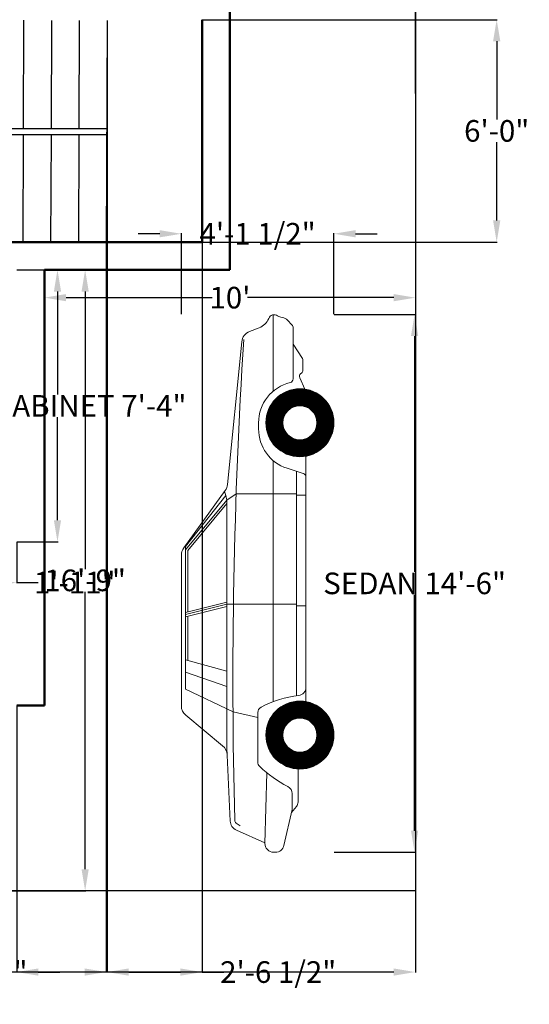
# Model space of a CAD drawing. Units: inches. Extents: x 164 to 612, y 17 to 606.
# Tile 2 of 3: x 448 to 612, y 17 to 335. Entities that reach past the tile are written whole.
import ezdxf

# ---------------------------------------------------------------- set-up
doc = ezdxf.new("R2010")
doc.units = ezdxf.units.IN
doc.header["$MEASUREMENT"] = 0
for name, color, linetype, lineweight in [('A-ANNO-DIMS', 2, 'Continuous', 18), ('A-FLOR-STRS', 7, 'Continuous', 25), ('A-WALL', 7, 'Continuous', 50), ('C-PRKG-VEHI', 8, 'Continuous', 18), ('C-PROP', 3, 'Continuous', 25)]:
    doc.layers.add(name, color=color, linetype=linetype, lineweight=lineweight)
doc.styles.get("Standard").update_dxf_attribs({"font": 'arial.ttf'})
doc.dimstyles.get("Standard").update_dxf_attribs({"dimtxt": 7, "dimasz": 7, "dimexe": 0.18, "dimexo": 0.0625, "dimgap": 0.09, "dimtad": 0, "dimtih": 1, "dimtoh": 1, "dimdec": 0, "dimzin": 0, "dimdsep": 46, "dimlunit": 3, "dimtxsty": 'Standard', "dimcen": 0.09, "dimadec": 0, "dimazin": 0, "dimtfac": 1, "dimtdec": 0, "dimtofl": 0, "dimtmove": 0, "dimatfit": 3, "dimfxl": 1, "dimtolj": 1, "dimtzin": 0, "dimarcsym": 0})

# ---------------------------------------------------------------- blocks, each defined once
blk = doc.blocks.new('Car - sedan  side')
for p, q in [((-139.53, 35.99), (-129.64, 47.91)), ((-128.57, 32.64), (-121.22, 48.02)), ((-77.81, 49.34), (-126.58, 49.34)), ((-74.7, 48.02), (-121.22, 48.02)), ((-120.32, 34.67), (-115.67, 48.02)), ((-115.4, 34.67), (-111.74, 48.02)), ((-94.41, 34.67), (-97.73, 48.02)), ((-93.72, 34.67), (-97.04, 48.02)), ((-93.03, 34.67), (-96.34, 48.02)), ((-60.02, 34.65), (-76.07, 48.02)), ((-56.87, 35.13), (-75.48, 48.59)), ((-58.54, 34.93), (-74.99, 48.02)), ((-97.55, 47.3), (-111.94, 47.3)), ((-76.26, 47.3), (-96.16, 47.3)), ((-61.08, 34.66), (-76.26, 47.3)), ((-57.21, 35.38), (-58.54, 34.93)), ((-140.23, 34.67), (-163.88, 33.56)), ((-62.28, 34.67), (-140.23, 34.67)), ((-130.39, 24.63), (-128.57, 32.64)), ((-93.72, 19.62), (-93.72, 34.67)), ((-62.28, 34.67), (-60.02, 34.65)), ((-60.02, 34.65), (-58.54, 34.93)), ((-57.97, 31.61), (-60.02, 34.65)), ((-54.93, 34.4), (-8.75, 29.8)), ((-170.93, 22.32), (-166.81, 31.56)), ((-164.57, 31.6), (-165.48, 30.35)), ((-57.97, 19.62), (-57.97, 31.61)), ((-4.21, 24.18), (-5.42, 27.27)), ((-148.26, 21.7), (-171.11, 22.33)), ((-128.78, 24.63), (-144.79, 24.63)), ((-36.97, 24.38), (-34.94, 24.38)), ((-174, 19.51), (-174, 18.91)), ((-47.2, 19.62), (-125.23, 19.62)), ((-93.72, 12.14), (-93.72, 19.62)), ((-57.97, 12.14), (-57.97, 19.62)), ((0, 19.62), (-24.7, 19.62)), ((-160.12, 13.48), (-171.81, 16.16)), ((-159.22, 12.14), (-161.08, 13.7)), ((-155.01, 13.48), (-160.12, 13.48)), ((-51.4, 9.89), (-49.69, 15.14)), ((-4.23, 13.19), (-20.72, 13.19)), ((-9.5, 13.19), (-14.1, 10.2)), ((-3.22, 13.59), (-1.77, 14.97)), ((-147.03, 11.6), (-157.73, 11.6)), ((-50.67, 12.14), (-123.32, 12.14)), ((-94.21, 9.03), (-94.21, 12.14)), ((-58.39, 9.03), (-58.39, 12.14)), ((-20.36, 11.06), (-24.06, 9.44)), ((-18.83, 10.42), (-19.11, 10.76)), ((-14.68, 10.03), (-18.01, 10.03)), ((-120.62, 9.03), (-125.23, 9.03)), ((-45.76, 9.03), (-120.62, 9.03))]:
    blk.add_line(p, q)
at = {"const_width": 5.49}
for points in [[(-127.8, 11, -1), (-144.3, 11, -1)], [(-26.69, 11, -1), (-43.19, 11, -1)]]:
    blk.add_lwpolyline(points, format="xyb", close=True, dxfattribs=at)
for centre, radius in [((-136.05, 11), 11), ((-34.94, 11), 11), ((-136.05, 11), 5.51), ((-34.94, 11), 5.51)]:
    blk.add_circle(centre, radius)
for centre, radius, start, end in [((-126.58, 45.38), 3.97, 90, 140.3029), ((-77.81, 45.38), 3.97, 54.135, 90), ((-142.58, 38.53), 3.97, 272.6827, 320.3029), ((-54.54, 38.35), 3.97, 234.135, 264.3123), ((-163.72, 30.18), 3.38, 92.6827, 155.9736), ((-163.62, 30.91), 1.17, 91.491, 143.9553), ((-118.51, -1702.12), 1734.79, 86.34698, 91.49105), ((-9.15, 25.82), 4, 21.3107, 84.3123), ((-171.18, 19.51), 2.82, 88.4193, 180), ((-118.09, -2.78), 38.85, 136.3964, 152.9097), ((-144.79, 22.64), 1.98, 90, 136.3964), ((-128.78, 22.64), 1.98, 28.1371, 90), ((-157.14, 7.48), 34.14, 6.5135, 28.1371), ((-36.97, 11), 13.38, 90, 161.9732), ((-34.94, 11), 13.38, 13.5864, 90), ((0.9, 26.18), 5.49, 201.3107, 247.7048), ((-1.92, 19.3), 1.94, 325.3744, 67.7048), ((-171.18, 18.91), 2.82, 180, 257.0905), ((-3.82, 17.12), 2.96, 313.7173, 352.3839), ((2.46, 16.28), 3.37, 145.3744, 172.3839), ((-155.01, 16.1), 2.62, 270, 332.9097), ((-20.72, 14.43), 1.24, 193.5864, 270), ((-4.23, 14.65), 1.46, 270, 313.7173), ((-157.73, 13.93), 2.32, 230.1291, 270), ((-120.62, 11.65), 2.62, 186.5135, 270), ((-52.58, 10.27), 1.24, 270, 341.9732), ((-19.93, 10.09), 1.06, 39.301, 113.7159), ((-18.01, 11.09), 1.06, 219.301, 270), ((-14.68, 11.09), 1.06, 270, 303.047)]:
    blk.add_arc(centre, radius, start, end)
blk = doc.blocks.new('*D16')
at = {"layer": 'A-ANNO-DIMS', "color": 0, "lineweight": -2, "transparency": 16777216}
for p, q in [((575.57, 311.32), (575.57, 245.22)), ((455.57, 254.32), (455.57, 245.22)), ((462.57, 245.4), (509.87, 245.4)), ((568.57, 245.4), (521.27, 245.4))]:
    blk.add_line(p, q, dxfattribs=at)
at = {"layer": 'A-ANNO-DIMS', "color": 0, "transparency": 16777216}
for points in [[(462.57, 246.56), (462.57, 244.23), (455.57, 245.4)], [(568.57, 246.56), (568.57, 244.23), (575.57, 245.4)]]:
    blk.add_solid(points, dxfattribs=at)
at = {"layer": 'Defpoints', "color": 0, "transparency": 16777216}
for p in [(575.57, 311.38), (455.57, 254.38), (575.57, 245.4)]:
    blk.add_point(p, dxfattribs=at)
at = {"layer": 'A-ANNO-DIMS', "color": 0, "transparency": 16777216, "insert": (515.57, 245.4), "char_height": 7, "attachment_point": 5}
blk.add_mtext("\\A1;10'", dxfattribs=at)
blk = doc.blocks.new('*D17')
at = {"layer": 'A-ANNO-DIMS', "color": 0, "lineweight": -2, "transparency": 16777216}
for p, q in [((481.01, 254.38), (468.54, 254.38)), ((468.72, 247.38), (468.72, 157.54)), ((468.72, 60.38), (468.72, 150.22)), ((389.63, 53.38), (468.9, 53.38))]:
    blk.add_line(p, q, dxfattribs=at)
at = {"layer": 'A-ANNO-DIMS', "color": 0, "transparency": 16777216}
for points in [[(467.56, 247.38), (469.89, 247.38), (468.72, 254.38)], [(467.56, 60.38), (469.89, 60.38), (468.72, 53.38)]]:
    blk.add_solid(points, dxfattribs=at)
at = {"layer": 'Defpoints', "color": 0, "transparency": 16777216}
for p in [(481.07, 254.38), (389.57, 53.38), (468.72, 53.38)]:
    blk.add_point(p, dxfattribs=at)
at = {"layer": 'A-ANNO-DIMS', "color": 0, "transparency": 16777216, "insert": (468.72, 153.88), "char_height": 7, "attachment_point": 5}
blk.add_mtext('\\A1;16\'-9"', dxfattribs=at)
blk = doc.blocks.new('*D19')
at = {"layer": 'A-ANNO-DIMS', "color": 0, "lineweight": -2, "transparency": 16777216}
for p, q in [((506.57, 344.44), (506.57, 358.56)), ((513.57, 358.38), (531.68, 358.38)), ((568.57, 358.38), (550.46, 358.38)), ((575.57, 311.44), (575.57, 358.56))]:
    blk.add_line(p, q, dxfattribs=at)
at = {"layer": 'A-ANNO-DIMS', "color": 0, "transparency": 16777216}
for points in [[(513.57, 359.55), (513.57, 357.22), (506.57, 358.38)], [(568.57, 359.55), (568.57, 357.22), (575.57, 358.38)]]:
    blk.add_solid(points, dxfattribs=at)
at = {"layer": 'Defpoints', "color": 0, "transparency": 16777216}
for p in [(575.57, 358.38), (506.57, 344.38), (575.57, 311.38)]:
    blk.add_point(p, dxfattribs=at)
at = {"layer": 'A-ANNO-DIMS', "color": 0, "transparency": 16777216, "insert": (541.07, 358.38), "char_height": 7, "attachment_point": 5}
blk.add_mtext('\\A1;5\'-9"', dxfattribs=at)
blk = doc.blocks.new('*D30')
at = {"layer": 'A-ANNO-DIMS', "color": 0, "lineweight": -2, "transparency": 16777216}
for p, q in [((446.63, 254.38), (459.95, 254.38)), ((459.77, 247.38), (459.77, 214.08)), ((459.77, 173.36), (459.77, 206.66)), ((446.63, 166.36), (459.95, 166.36))]:
    blk.add_line(p, q, dxfattribs=at)
at = {"layer": 'A-ANNO-DIMS', "color": 0, "transparency": 16777216}
for points in [[(458.61, 247.38), (460.94, 247.38), (459.77, 254.38)], [(458.61, 173.36), (460.94, 173.36), (459.77, 166.36)]]:
    blk.add_solid(points, dxfattribs=at)
at = {"layer": 'Defpoints', "color": 0, "transparency": 16777216}
for p in [(446.57, 254.38), (459.77, 254.38), (446.57, 166.36)]:
    blk.add_point(p, dxfattribs=at)
at = {"layer": 'A-ANNO-DIMS', "color": 0, "transparency": 16777216, "insert": (459.77, 210.37), "char_height": 7, "attachment_point": 5}
blk.add_mtext('\\A1;FILE CABINET 7\'-4"', dxfattribs=at)
blk = doc.blocks.new('*D31')
at = {"layer": 'A-ANNO-DIMS', "color": 0, "lineweight": -2, "transparency": 16777216}
for p, q in [((423.41, 166.29), (423.41, 152.97)), ((446.57, 166.29), (446.57, 152.97)), ((430.41, 153.15), (439.57, 153.15)), ((446.57, 153.15), (453.57, 153.15))]:
    blk.add_line(p, q, dxfattribs=at)
at = {"layer": 'A-ANNO-DIMS', "color": 0, "transparency": 16777216}
for points in [[(430.41, 154.32), (430.41, 151.99), (423.41, 153.15)], [(439.57, 154.32), (439.57, 151.99), (446.57, 153.15)]]:
    blk.add_solid(points, dxfattribs=at)
at = {"layer": 'Defpoints', "color": 0, "transparency": 16777216}
for p in [(423.41, 166.36), (446.57, 166.36), (446.57, 153.15)]:
    blk.add_point(p, dxfattribs=at)
at = {"layer": 'A-ANNO-DIMS', "color": 0, "transparency": 16777216, "insert": (465.35, 153.15), "char_height": 7, "attachment_point": 5}
blk.add_mtext('\\A1;1\'-11"', dxfattribs=at)
blk = doc.blocks.new('*D36')
at = {"layer": 'A-ANNO-DIMS', "color": 0, "lineweight": -2, "transparency": 16777216}
for p, q in [((549.26, 239.97), (575.49, 239.97)), ((575.31, 232.97), (575.31, 156.62)), ((575.31, 72.85), (575.31, 149.2)), ((549.26, 65.85), (575.49, 65.85))]:
    blk.add_line(p, q, dxfattribs=at)
at = {"layer": 'A-ANNO-DIMS', "color": 0, "transparency": 16777216}
for points in [[(574.15, 232.97), (576.48, 232.97), (575.31, 239.97)], [(574.15, 72.85), (576.48, 72.85), (575.31, 65.85)]]:
    blk.add_solid(points, dxfattribs=at)
at = {"layer": 'Defpoints', "color": 0, "transparency": 16777216}
for p in [(549.2, 239.97), (575.31, 239.97), (549.2, 65.85)]:
    blk.add_point(p, dxfattribs=at)
at = {"layer": 'A-ANNO-DIMS', "color": 0, "transparency": 16777216, "insert": (575.31, 152.91), "char_height": 7, "attachment_point": 5}
blk.add_mtext('\\A1;SEDAN 14\'-6"', dxfattribs=at)
blk = doc.blocks.new('*D37')
at = {"layer": 'A-ANNO-DIMS', "color": 0, "lineweight": -2, "transparency": 16777216}
for p, q in [((492.85, 266.08), (485.85, 266.08)), ((499.85, 240.03), (499.85, 266.26)), ((549.2, 240.03), (549.2, 266.26)), ((556.2, 266.08), (563.2, 266.08))]:
    blk.add_line(p, q, dxfattribs=at)
at = {"layer": 'A-ANNO-DIMS', "color": 0, "transparency": 16777216}
for points in [[(492.85, 267.25), (492.85, 264.92), (499.85, 266.08)], [(556.2, 267.25), (556.2, 264.92), (549.2, 266.08)]]:
    blk.add_solid(points, dxfattribs=at)
at = {"layer": 'Defpoints', "color": 0, "transparency": 16777216}
for p in [(499.85, 266.08), (499.85, 239.97), (549.2, 239.97)]:
    blk.add_point(p, dxfattribs=at)
at = {"layer": 'A-ANNO-DIMS', "color": 0, "transparency": 16777216, "insert": (524.52, 266.08), "char_height": 7, "attachment_point": 5}
blk.add_mtext('\\A1;4\'-1 1/2"', dxfattribs=at)
blk = doc.blocks.new('*D42')
at = {"layer": 'A-ANNO-DIMS', "color": 0, "lineweight": -2, "transparency": 16777216}
for p, q in [((203.57, 53.32), (203.57, 26.9)), ((575.57, 53.32), (575.57, 26.9)), ((210.57, 27.08), (377.46, 27.08)), ((568.57, 27.08), (401.68, 27.08))]:
    blk.add_line(p, q, dxfattribs=at)
at = {"layer": 'A-ANNO-DIMS', "color": 0, "transparency": 16777216}
for points in [[(210.57, 28.25), (210.57, 25.91), (203.57, 27.08)], [(568.57, 28.25), (568.57, 25.91), (575.57, 27.08)]]:
    blk.add_solid(points, dxfattribs=at)
at = {"layer": 'Defpoints', "color": 0, "transparency": 16777216}
for p in [(203.57, 53.38), (575.57, 53.38), (575.57, 27.08)]:
    blk.add_point(p, dxfattribs=at)
at = {"layer": 'A-ANNO-DIMS', "color": 0, "transparency": 16777216, "insert": (389.57, 27.08), "char_height": 7, "attachment_point": 5}
blk.add_mtext('\\A1;31\'-0"', dxfattribs=at)
blk = doc.blocks.new('*D48')
at = {"layer": 'A-ANNO-DIMS', "color": 0, "lineweight": -2, "transparency": 16777216}
for p, q in [((414.57, 113.32), (414.57, 26.9)), ((446.57, 113.32), (446.57, 26.9)), ((407.57, 27.08), (400.57, 27.08)), ((453.57, 27.08), (460.57, 27.08))]:
    blk.add_line(p, q, dxfattribs=at)
at = {"layer": 'A-ANNO-DIMS', "color": 0, "transparency": 16777216}
for points in [[(407.57, 28.25), (407.57, 25.91), (414.57, 27.08)], [(453.57, 28.25), (453.57, 25.91), (446.57, 27.08)]]:
    blk.add_solid(points, dxfattribs=at)
at = {"layer": 'Defpoints', "color": 0, "transparency": 16777216}
for p in [(414.57, 113.38), (446.57, 113.38), (446.57, 27.08)]:
    blk.add_point(p, dxfattribs=at)
at = {"layer": 'A-ANNO-DIMS', "color": 0, "transparency": 16777216, "insert": (430.57, 27.08), "char_height": 7, "attachment_point": 5}
blk.add_mtext('\\A1;2\'-8"', dxfattribs=at)
blk = doc.blocks.new('*D51')
at = {"layer": 'A-ANNO-DIMS', "color": 0, "lineweight": -2, "transparency": 16777216}
for p, q in [((506.63, 335.38), (602.05, 335.38)), ((601.87, 328.38), (601.87, 303.04)), ((601.87, 270.38), (601.87, 295.72)), ((506.63, 263.38), (602.05, 263.38))]:
    blk.add_line(p, q, dxfattribs=at)
at = {"layer": 'A-ANNO-DIMS', "color": 0, "transparency": 16777216}
for points in [[(600.7, 328.38), (603.04, 328.38), (601.87, 335.38)], [(600.7, 270.38), (603.04, 270.38), (601.87, 263.38)]]:
    blk.add_solid(points, dxfattribs=at)
at = {"layer": 'Defpoints', "color": 0, "transparency": 16777216}
for p in [(506.57, 335.38), (601.87, 335.38), (506.57, 263.38)]:
    blk.add_point(p, dxfattribs=at)
at = {"layer": 'A-ANNO-DIMS', "color": 0, "transparency": 16777216, "insert": (601.87, 299.38), "char_height": 7, "attachment_point": 5}
blk.add_mtext('\\A1;6\'-0"', dxfattribs=at)
blk = doc.blocks.new('*D52')
at = {"layer": 'A-ANNO-DIMS', "color": 0, "lineweight": -2, "transparency": 16777216}
for p, q in [((403.53, 263.32), (403.53, 26.9)), ((475.53, 263.01), (475.53, 26.9)), ((410.53, 27.08), (430.12, 27.08)), ((468.53, 27.08), (448.95, 27.08))]:
    blk.add_line(p, q, dxfattribs=at)
at = {"layer": 'A-ANNO-DIMS', "color": 0, "transparency": 16777216}
for points in [[(410.53, 28.25), (410.53, 25.91), (403.53, 27.08)], [(468.53, 28.25), (468.53, 25.91), (475.53, 27.08)]]:
    blk.add_solid(points, dxfattribs=at)
at = {"layer": 'Defpoints', "color": 0, "transparency": 16777216}
for p in [(403.53, 263.38), (475.53, 263.08), (475.53, 27.08)]:
    blk.add_point(p, dxfattribs=at)
at = {"layer": 'A-ANNO-DIMS', "color": 0, "transparency": 16777216, "insert": (439.53, 27.08), "char_height": 7, "attachment_point": 5}
blk.add_mtext('\\A1;6\'-0"', dxfattribs=at)
blk = doc.blocks.new('*D53')
at = {"layer": 'A-ANNO-DIMS', "color": 0, "lineweight": -2, "transparency": 16777216}
for p, q in [((475.83, 335.01), (475.83, 26.9)), ((506.57, 335.32), (506.57, 26.9)), ((482.83, 27.08), (499.57, 27.08)), ((506.57, 27.08), (513.57, 27.08))]:
    blk.add_line(p, q, dxfattribs=at)
at = {"layer": 'A-ANNO-DIMS', "color": 0, "transparency": 16777216}
for points in [[(482.83, 28.25), (482.83, 25.91), (475.83, 27.08)], [(499.57, 28.25), (499.57, 25.91), (506.57, 27.08)]]:
    blk.add_solid(points, dxfattribs=at)
at = {"layer": 'Defpoints', "color": 0, "transparency": 16777216}
for p in [(475.83, 335.08), (506.57, 335.38), (506.57, 27.08)]:
    blk.add_point(p, dxfattribs=at)
at = {"layer": 'A-ANNO-DIMS', "color": 0, "transparency": 16777216, "insert": (531.18, 27.08), "char_height": 7, "attachment_point": 5}
blk.add_mtext('\\A1;2\'-6 1/2"', dxfattribs=at)

msp = doc.modelspace()

# ---------------------------------------------------------------- linework, layer by layer
at = {"layer": 'A-FLOR-STRS'}
for p, q in [((448.83, 335.19), (448.69, 300.08)), ((457.83, 335.15), (457.69, 300.08)), ((466.83, 335.11), (466.69, 300.08)), ((475.83, 335.08), (475.53, 263.08)), ((475.68, 300.08), (403.68, 300.08)), ((475.68, 298.08), (403.68, 298.08)), ((448.68, 298.08), (448.53, 263.19)), ((457.68, 298.08), (457.53, 263.15)), ((466.68, 298.08), (466.53, 263.11))]:
    msp.add_line(p, q, dxfattribs=at)
at = {"layer": 'A-WALL'}
for p, q in [((515.57, 521.38), (515.57, 254.38)), ((506.57, 335.38), (506.57, 263.38)), ((392.57, 263.38), (506.57, 263.38)), ((455.57, 122.38), (455.57, 254.38)), ((455.57, 254.38), (506.57, 254.38)), ((506.57, 254.38), (515.57, 254.38)), ((455.57, 122.38), (455.57, 113.38)), ((455.57, 113.38), (446.57, 113.38))]:
    msp.add_line(p, q, dxfattribs=at)
at = {"layer": 'C-PROP'}
for p, q in [((575.57, 569.38), (575.57, 53.38)), ((575.57, 53.38), (203.57, 53.38))]:
    msp.add_line(p, q, dxfattribs=at)

# ---------------------------------------------------------------- block references
at = {"layer": 'C-PRKG-VEHI', "rotation": 90}
msp.add_blockref('Car - sedan  side', (549.2, 239.85), dxfattribs=at)

# ---------------------------------------------------------------- dimensions: what is measured, and where the dimension line sits
at = {"layer": 'A-ANNO-DIMS'}
for base, p1, p2, override, picture, middle in [((575.57, 358.38), (506.57, 344.38), (575.57, 311.38), {"dimclrd": 0, "dimclre": 0, "dimclrt": 0}, '*D19', (541.07, 358.38)), ((506.57, 27.08), (475.83, 335.08), (506.57, 335.38), {"dimdec": 1, "dimlfac": 1, "dimrnd": 0, "dimzin": 1, "dimdsep": 46, "dimlunit": 4, "dimfrac": 2}, '*D53', (531.18, 27.08)), ((575.57, 245.4), (455.57, 254.38), (575.57, 311.38), {"dimclrd": 0, "dimclre": 0, "dimclrt": 0}, '*D16', (515.57, 245.4)), ((475.53, 27.08), (403.53, 263.38), (475.53, 263.08), {"dimdec": 1, "dimlfac": 1, "dimrnd": 0, "dimzin": 1, "dimdsep": 46, "dimlunit": 4, "dimfrac": 2}, '*D52', (439.53, 27.08)), ((446.57, 153.15), (423.41, 166.36), (446.57, 166.36), {"dimdec": 1, "dimlfac": 1, "dimrnd": 0, "dimzin": 1, "dimdsep": 46, "dimlunit": 4, "dimfrac": 2}, '*D31', (465.35, 153.15)), ((446.57, 27.08), (414.57, 113.38), (446.57, 113.38), {"dimdec": 1, "dimlfac": 1, "dimrnd": 0, "dimzin": 1, "dimdsep": 46, "dimlunit": 4, "dimfrac": 2}, '*D48', (430.57, 27.08)), ((575.57, 27.08), (203.57, 53.38), (575.57, 53.38), {"dimdec": 1, "dimlfac": 1, "dimrnd": 0, "dimzin": 1, "dimdsep": 46, "dimlunit": 4, "dimfrac": 2}, '*D42', (389.57, 27.08))]:
    dim = msp.add_linear_dim(base=base, p1=p1, p2=p2, dimstyle='Standard', override=override, dxfattribs=at)
    dim.commit()
    dim.dimension.update_dxf_attribs({"geometry": picture, "text_midpoint": middle})
for base, p1, p2, angle, override, picture, middle in [((601.87, 335.38), (506.57, 263.38), (506.57, 335.38), 90, {"dimdec": 1, "dimlfac": 1, "dimrnd": 0, "dimzin": 1, "dimdsep": 46, "dimlunit": 4, "dimfrac": 2}, '*D51', (601.87, 299.38)), ((499.8514, 266.0826), (549.1963, 239.9656), (499.8514, 239.9656), 180, {"dimdec": 1, "dimlfac": 1, "dimrnd": 0, "dimzin": 1, "dimdsep": 46, "dimlunit": 4, "dimfrac": 2}, '*D37', (524.5239, 266.0826)), ((468.72, 53.38), (481.07, 254.38), (389.57, 53.38), 90, {"dimclrd": 0, "dimclre": 0, "dimclrt": 0}, '*D17', (468.72, 153.88))]:
    dim = msp.add_linear_dim(base=base, p1=p1, p2=p2, angle=angle, dimstyle='Standard', override=override, dxfattribs=at)
    dim.commit()
    dim.dimension.update_dxf_attribs({"geometry": picture, "text_midpoint": middle})
for base, p1, p2, text, picture, middle in [((459.77, 254.38), (446.57, 166.36), (446.57, 254.38), 'FILE CABINET <>', '*D30', (459.77, 210.37)), ((575.31, 239.97), (549.2, 65.85), (549.2, 239.97), 'SEDAN <>', '*D36', (575.31, 152.91))]:
    dim = msp.add_linear_dim(base=base, p1=p1, p2=p2, angle=90, text=text, dimstyle='Standard', override={"dimdec": 1, "dimlfac": 1, "dimrnd": 0, "dimzin": 1, "dimdsep": 46, "dimlunit": 4, "dimfrac": 2}, dxfattribs=at)
    dim.commit()
    dim.dimension.update_dxf_attribs({"geometry": picture, "text_midpoint": middle})

doc.saveas('drawing.dxf')
